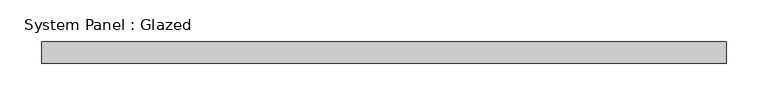
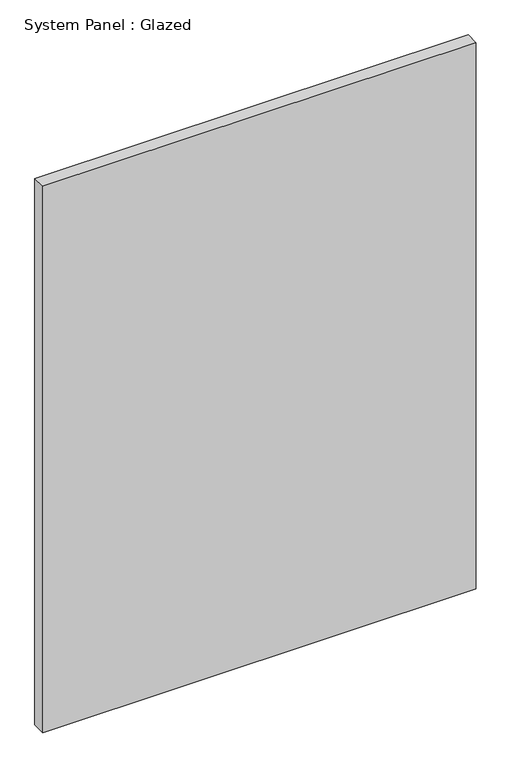
"""IFC4 building model written with IfcOpenShell, lengths in millimetres: plate geometry, System Panel : Glazed."""

from ifc_helpers import new_model, si_unit, origin, origin_with_axes, place, context, project, spatial, polyline, outline, extrude, source, transform, mapped, element, save


def system_panel_glazed_cc4caca5(model_context):
    return source(origin(), model_context, "Body", "SweptSolid", [
        extrude(outline(polyline([(409.575, -44.45), (-409.575, -44.45), (-409.575, -19.05), (409.575, -19.05), (409.575, -44.45)])), origin_with_axes(), (0.0, 0.0, 1.0), 1092.2),
    ])


if __name__ == "__main__":
    model = new_model("IFC4")
    model_context = context("Model", 3, world=origin())
    ifc_project = project(units=[si_unit("LENGTHUNIT", "METRE", prefix="MILLI")], contexts=[model_context])
    site = spatial("IfcSite", under=ifc_project)
    building = spatial("IfcBuilding", under=site)
    placement = place(None, origin())
    system_panel_glazed_shape = system_panel_glazed_cc4caca5(model_context)
    element("IfcPlate", 1, ObjectType="System Panel : Glazed", at=placement, inside=building, context=model_context, shape_type="MappedRepresentation", body=[
        mapped(system_panel_glazed_shape, transform((0.0, 0.0, 0.0), x_axis=(1.0, 0.0, 0.0), y_axis=(0.0, 1.0, 0.0), z_axis=(0.0, 0.0, 1.0))),
    ])
    save(model, "model.ifc")

# Revit data of these elements
# Type "System Panel : Glazed"
#   Construction Type Id = "GSP4R"
#   Analytic Construction = "1/8 in Pilkington single glazing"
#   Visual Light Transmittance = 0.9
#   Solar Heat Gain Coefficient = 0.86
#   Heat Transfer Coefficient (U) = 1.18115 BTU/(h·ft²·°F)
#   Define Thermal Properties by = 1
# Element 1 (IfcPlate, "System Panel : Glazed")
#   Materials on its faces: "Glass"
# Materials
#   "Glass": class "Glass", colour RGB 0 128 192, transparency 0.75, Description = "Soda Lime Glass", Cost = 0
